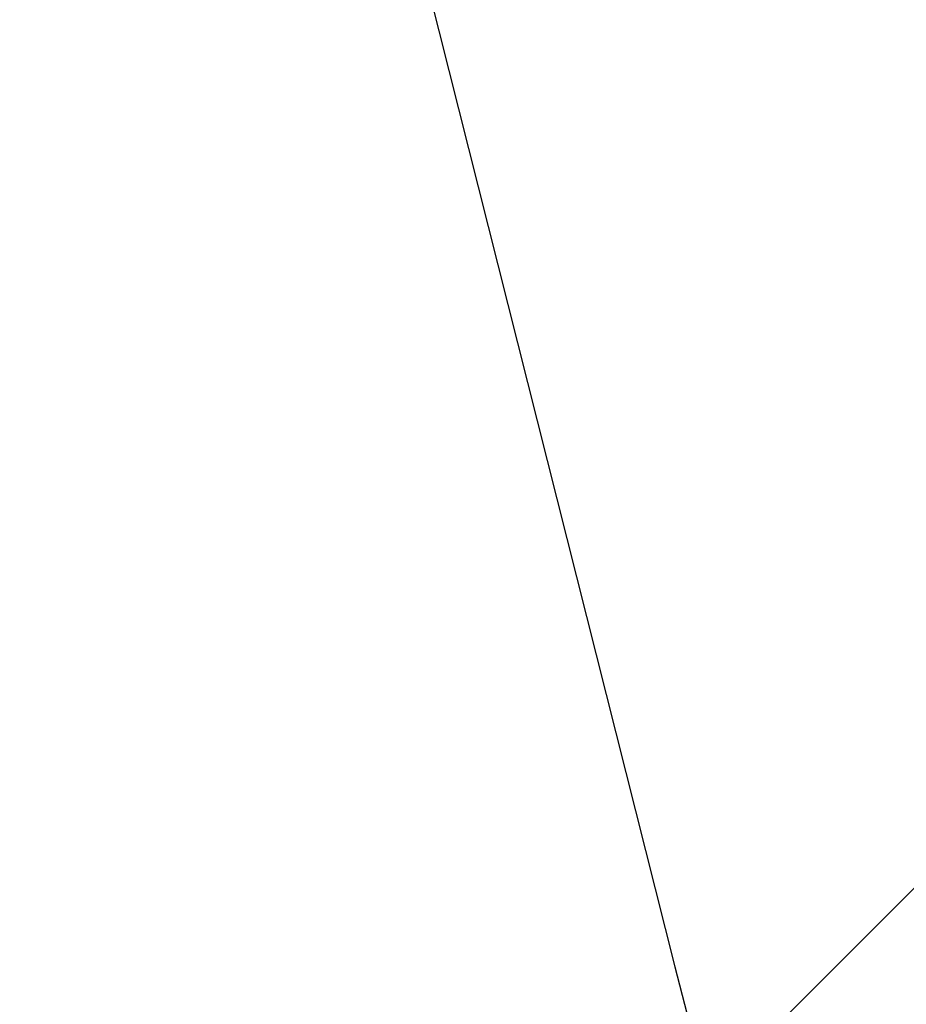
# Model space of a CAD drawing. Units: inches. Extents: x 3590 to 5167, y 65 to 1917.
# Tile 77 of 100: x 5047.497 to 5049.155, y 1787.19 to 1789.032. Entities that reach past the tile are written whole.
import ezdxf

# ---------------------------------------------------------------- set-up
doc = ezdxf.new("R2010")
doc.units = ezdxf.units.IN
for name, color, linetype, lineweight in [('A-ANNO-DIMS', 2, 'Continuous', 18), ('A-FLOR-PATT', 8, 'Continuous', 13), ('L-PLNT', 94, 'Continuous', 18)]:
    doc.layers.add(name, color=color, linetype=linetype, lineweight=lineweight)
doc.layers.add('DIENHOA', color=3, linetype='Continuous')
doc.styles.get("Standard").update_dxf_attribs({"font": 'arial.ttf'})
doc.dimstyles.new('ISO-25', dxfattribs={"dimtxt": 9, "dimasz": 2.5, "dimexe": 1.25, "dimexo": 0.625, "dimtad": 1, "dimdec": 1, "dimlunit": 3, "dimtxsty": 'Standard', "dimcen": 2.5, "dimadec": 0, "dimazin": 0, "dimtfac": 1, "dimtdec": 1, "dimtmove": 0, "dimatfit": 3, "dimfxl": 1, "dimarcsym": 0})

# ---------------------------------------------------------------- blocks, each defined once
blk = doc.blocks.new('Cay03_mb')
at = {"layer": 'DIENHOA'}
blk.add_lwpolyline([(-156.54, 633.124), (-132.463, 551.333), (-110.511, 470.016), (-89.843, 389.218), (-69.618, 308.982), (-48.993, 229.354), (-27.129, 150.379), (-3.182, 72.099), (23.687, -5.439)], dxfattribs=at)
blk = doc.blocks.new('*D322')
at = {"layer": 'A-ANNO-DIMS', "color": 0, "lineweight": -2, "transparency": 16777216}
for p, q in [((5035.7437, 1766.1842), (5035.7437, 1761.199)), ((5064.812, 1766.1842), (5064.812, 1761.199)), ((5038.2437, 1762.449), (5062.312, 1762.449)), ((5064.812, 1762.449), (5166.9911, 1762.449))]:
    blk.add_line(p, q, dxfattribs=at)
at = {"layer": 'A-ANNO-DIMS', "color": 0, "transparency": 16777216}
for points in [[(5038.2437, 1762.8657), (5038.2437, 1762.0323), (5035.7437, 1762.449)], [(5062.312, 1762.8657), (5062.312, 1762.0323), (5064.812, 1762.449)]]:
    blk.add_solid(points, dxfattribs=at)
at = {"layer": 'Defpoints', "color": 0, "transparency": 16777216}
for p in [(5035.7437, 1766.8092), (5064.812, 1766.8092), (5064.812, 1762.449)]:
    blk.add_point(p, dxfattribs=at)
at = {"layer": 'A-ANNO-DIMS', "color": 0, "transparency": 16777216, "insert": (5117.1516, 1767.6692), "char_height": 9, "attachment_point": 5}
blk.add_mtext('PLANT 2\'-5" TYP.', dxfattribs=at)

msp = doc.modelspace()

# ---------------------------------------------------------------- hatches: boundary and pattern name
at = {"layer": 'A-FLOR-PATT', "transparency": 33554687}
h = msp.add_hatch(dxfattribs=at)
h.set_pattern_fill('AR-HBONE', color=256, scale=0.2)
h.set_pattern_definition([(45, (-588.972, 0), (0, 28.73682), [60.96, -20.32]), (135, (-574.604, 14.368), (3e-15, 28.73682), [60.96, -20.32])])
h.paths.add_polyline_path([(5071.274, 1796.999), (4933.274, 1796.999), (4933.274, 1753.999), (4962.774, 1753.999, -0.414214), (4928.774, 1719.999), (4933.274, 1718.999), (4933.274, 1334.999), (5071.274, 1334.999)])
h.paths.add_polyline_path([(4951.78, 1521.0767), (4951.7151, 1521.0404), (4951.5634, 1520.8953)], flags=16)
h.paths.add_polyline_path([(4952.267, 1521.3764), (4952.1977, 1521.3711), (4952.1982, 1521.3556)], flags=0)
h.paths.add_polyline_path([(4967.0508, 1529.7283), (4965.2312, 1528.6944), (4963.4111, 1527.714), (4961.7565, 1526.8508), (4963.5889, 1527.4494), (4964.0356, 1527.478), (4962.9755, 1527.249), (4961.7602, 1526.852), (4959.7922, 1525.8341), (4958.005, 1524.8948), (4956.2403, 1523.9296), (4954.5039, 1522.9185), (4954.1294, 1522.6816), (4953.3605, 1521.9969), (4953.3656, 1521.9975), (4953.605, 1522.0637), (4955.1061, 1522.7608), (4956.9211, 1523.4341), (4958.6778, 1523.9151), (4960.3583, 1524.2004), (4961.9446, 1524.2861), (4964.1714, 1524.1085), (4965.9575, 1523.309), (4963.8627, 1522.9756), (4965.1874, 1522.499), (4963.3661, 1522.4971), (4961.5453, 1522.4868), (4959.7636, 1522.4608), (4958.3041, 1522.4188), (4957.9736, 1522.3883), (4956.3069, 1522.2324), (4954.7182, 1522.0714), (4953.2508, 1521.8992), (4953.5251, 1521.6228), (4954.3309, 1521.3788), (4956.2426, 1521.2299), (4958.0391, 1520.9295), (4959.6842, 1520.4834), (4961.1601, 1519.8957), (4963.107, 1518.8002), (4964.3929, 1517.3252), (4962.9731, 1517.726), (4964.5584, 1516.6606), (4965.4066, 1515.7078), (4963.5073, 1516.3218), (4961.68, 1517.0051), (4959.9348, 1517.7449), (4958.2821, 1518.5283), (4956.7322, 1519.3426), (4955.2953, 1520.1748), (4954.6715, 1520.5724), (4954.5128, 1520.6271), (4955.6585, 1519.3184), (4956.7026, 1517.9823), (4957.644, 1516.6466), (4958.4855, 1515.3344), (4959.55, 1513.524), (4960.4377, 1511.7694), (4958.8411, 1513.6196), (4957.4517, 1515.3249), (4955.8186, 1517.4586), (4956.6654, 1515.4476), (4957.1111, 1513.9229), (4957.4468, 1511.7143), (4957.0764, 1509.7929), (4956.5376, 1511.1103), (4955.9923, 1512.5689), (4955.4445, 1514.1251), (4954.8979, 1515.7352), (4954.3565, 1517.3555), (4953.8241, 1518.9425), (4953.3046, 1520.4525), (4953.0645, 1521.1156), (4952.9714, 1521.1461), (4952.9493, 1521.0865), (4952.7298, 1520.199), (4953.3698, 1518.0236), (4953.7571, 1516.3728), (4954.0512, 1514.7654), (4954.2645, 1513.2212), (4954.4712, 1511.1312), (4954.4971, 1510.4017), (4954.409, 1511.7601), (4954.2645, 1513.2212), (4954.0512, 1514.7654), (4953.7571, 1516.3728), (4953.3698, 1518.0236), (4952.8772, 1519.6981), (4952.7161, 1520.1412), (4952.533, 1519.0587), (4952.3743, 1517.7888), (4952.2192, 1516.3117), (4952.046, 1514.5999), (4951.8325, 1512.626), (4951.557, 1510.3626), (4951.2033, 1512.1682), (4950.8517, 1514.3393), (4950.9853, 1516.3759), (4951.6596, 1518.2862), (4952.5926, 1520.4808), (4952.3566, 1521.1299), (4951.855, 1520.3275), (4950.839, 1518.9083), (4949.7767, 1517.5866), (4948.9155, 1516.6173), (4948.111, 1515.2561), (4947.0891, 1513.5539), (4945.8894, 1511.6149), (4946.3259, 1513.4023), (4946.5624, 1514.2491), (4945.5277, 1513.3267), (4944.5811, 1512.5313), (4946.0177, 1514.5082), (4947.2044, 1516.0476), (4947.8933, 1517.3133), (4949.3069, 1518.7645), (4950.4142, 1519.7672), (4950.4513, 1519.8063), (4952.267, 1521.3764), (4951.6446, 1521.4932), (4950.4037, 1521.1795), (4948.0445, 1520.3587), (4946.1186, 1519.452), (4944.5718, 1518.4748), (4943.3496, 1517.4427), (4941.997, 1515.9197), (4941.6615, 1515.2748), (4942.8133, 1516.9897), (4944.5718, 1518.4748), (4946.1186, 1519.452), (4948.0445, 1520.3587), (4950.4037, 1521.1795), (4951.6446, 1521.4932), (4949.6468, 1521.8678), (4948.5998, 1521.7563), (4947.1263, 1521.5699), (4945.4202, 1521.3476), (4943.4497, 1521.1046), (4941.1832, 1520.856), (4942.8603, 1521.6126), (4943.8731, 1522.0301), (4942.9522, 1521.9093), (4941.4097, 1521.4851), (4939.5429, 1520.6702), (4938.9677, 1520.2255), (4940.7328, 1521.299), (4942.9522, 1521.9093), (4943.7018, 1522.0077), (4945.8942, 1522.7), (4947.5649, 1522.714), (4948.9209, 1522.5657), (4951.1314, 1522.1827), (4950.9706, 1522.2969), (4948.1292, 1523.0056), (4946.035, 1523.7067), (4944.2323, 1524.5214), (4942.7069, 1525.4611), (4941.4442, 1526.5371), (4940.4297, 1527.7606), (4939.6489, 1529.1431), (4941.4209, 1528.1223), (4943.1474, 1527.1325), (4944.8409, 1526.1746), (4946.5139, 1525.2496), (4948.1789, 1524.3586), (4948.3646, 1524.2634), (4946.4753, 1526.0446), (4945.1808, 1527.5404), (4944.1904, 1529.0334), (4943.4956, 1530.5398), (4943.2781, 1531.3597), (4942.4985, 1531.919), (4943.1135, 1531.7625), (4942.9593, 1533.6586), (4944.1395, 1531.9886), (4944.6117, 1531.3234), (4946.2016, 1530.4634), (4947.4857, 1529.5093), (4948.7903, 1528.2265), (4950.3675, 1526.2375), (4949.4855, 1528.1555), (4948.8513, 1530.1225), (4948.4905, 1532.0413), (4948.3811, 1533.9182), (4948.5006, 1535.7599), (4948.827, 1537.5728), (4949.418, 1535.5653), (4949.9568, 1533.5693), (4950.4641, 1531.5861), (4950.9606, 1529.6167), (4951.3911, 1527.9545), (4951.7235, 1530.6869), (4952.2011, 1532.5799), (4952.8891, 1534.3296), (4953.7703, 1535.9512), (4954.8273, 1537.46), (4954.5214, 1535.3897), (4954.2731, 1533.9368), (4955.58, 1535.6627), (4956.7476, 1536.7386), (4956.1585, 1534.7803), (4955.5892, 1532.8733), (4955.0434, 1531.0058), (4954.5249, 1529.1658), (4954.0377, 1527.3413), (4953.6383, 1525.733), (4953.6114, 1525.5856), (4953.3981, 1524.1657), (4953.3822, 1524.0089), (4954.0696, 1525.4756), (4954.9121, 1527.0217), (4956.1363, 1528.8935), (4957.8467, 1530.577), (4959.376, 1531.5401), (4958.256, 1530.104), (4957.1428, 1528.6629), (4956.0663, 1527.2431), (4955.0558, 1525.8705), (4954.141, 1524.5715), (4953.3516, 1523.372), (4953.3108, 1523.303), (4953.2725, 1522.9248), (4953.261, 1522.3821), (4954.1031, 1523.3727), (4954.63, 1524.2838), (4955.9615, 1526.3577), (4957.23, 1528.1297), (4958.4206, 1529.6086), (4960.0367, 1531.3679), (4961.3736, 1532.3752), (4962.1015, 1532.77), (4961.0699, 1531.0611), (4959.9873, 1529.4381), (4958.8685, 1527.908), (4958.1505, 1527.0074), (4959.8029, 1528.0031), (4961.5885, 1528.7926), (4963.3909, 1529.3278), (4965.2112, 1529.6321)], flags=16)
h.paths.add_polyline_path([(4962.9439, 1523.1819), (4961.1071, 1523.4219), (4960.3921, 1523.3616), (4962.3496, 1523.3306)], flags=0)
h.paths.add_polyline_path([(5049.5413, 1584.5509), (5049.4764, 1584.5146), (5049.3247, 1584.3695)], flags=16)
h.paths.add_polyline_path([(5050.0283, 1584.8506), (5049.959, 1584.8453), (5049.9595, 1584.8298)], flags=0)
h.paths.add_polyline_path([(5042.3331, 1581.949), (5043.8799, 1582.9262), (5045.8057, 1583.8329), (5048.165, 1584.6537), (5049.4058, 1584.9674), (5047.408, 1585.342), (5046.3611, 1585.2305), (5044.8876, 1585.0441), (5043.1814, 1584.8218), (5041.211, 1584.5788), (5038.9445, 1584.3301), (5040.6215, 1585.0868), (5041.6343, 1585.5043), (5040.7134, 1585.3835), (5039.1709, 1584.9593), (5037.3041, 1584.1444), (5036.729, 1583.6997), (5038.4941, 1584.7732), (5040.7134, 1585.3835), (5041.4631, 1585.4819), (5043.6555, 1586.1742), (5045.3261, 1586.1882), (5046.6821, 1586.0399), (5048.8927, 1585.6569), (5048.7319, 1585.7711), (5045.8905, 1586.4798), (5043.7962, 1587.1809), (5041.9936, 1587.9956), (5040.4682, 1588.9353), (5039.2055, 1590.0113), (5038.1909, 1591.2348), (5037.4102, 1592.6172), (5039.1822, 1591.5965), (5040.9087, 1590.6067), (5042.6022, 1589.6488), (5044.2752, 1588.7238), (5045.9402, 1587.8327), (5046.1258, 1587.7375), (5044.2366, 1589.5188), (5042.9421, 1591.0146), (5041.9517, 1592.5076), (5041.2569, 1594.014), (5041.0393, 1594.8339), (5040.2598, 1595.3932), (5040.8748, 1595.2367), (5040.7205, 1597.1328), (5041.9008, 1595.4628), (5042.373, 1594.7976), (5043.9629, 1593.9376), (5045.2469, 1592.9834), (5046.5515, 1591.7007), (5048.1288, 1589.7116), (5047.2467, 1591.6297), (5046.6125, 1593.5967), (5046.2518, 1595.5155), (5046.1423, 1597.3924), (5046.2619, 1599.2341), (5046.5883, 1601.047), (5047.1793, 1599.0394), (5047.7181, 1597.0435), (5048.2254, 1595.0603), (5048.7218, 1593.0909), (5049.1524, 1591.4287), (5049.4848, 1594.1611), (5049.9623, 1596.0541), (5050.6504, 1597.8038), (5051.5316, 1599.4254), (5052.5885, 1600.9341), (5052.2827, 1598.8638), (5052.0344, 1597.411), (5053.3413, 1599.1369), (5054.5088, 1600.2128), (5053.9198, 1598.2545), (5053.3504, 1596.3475), (5052.8046, 1594.48), (5052.2862, 1592.6399), (5051.799, 1590.8155), (5051.3996, 1589.2072), (5051.3727, 1589.0598), (5051.1593, 1587.6398), (5051.1435, 1587.4831), (5051.8308, 1588.9498), (5052.6734, 1590.4959), (5053.8975, 1592.3677), (5055.6079, 1594.0512), (5057.1373, 1595.0143), (5056.0172, 1593.5782), (5054.9041, 1592.1371), (5053.8275, 1590.7172), (5052.8171, 1589.3447), (5051.9023, 1588.0457), (5051.1129, 1586.8462), (5051.0721, 1586.7772), (5051.0338, 1586.399), (5051.0223, 1585.8563), (5051.8644, 1586.8469), (5052.3913, 1587.7579), (5053.7228, 1589.8318), (5054.9913, 1591.6039), (5056.1818, 1593.0828), (5057.798, 1594.8421), (5059.1349, 1595.8494), (5059.8628, 1596.2442), (5058.8312, 1594.5353), (5057.7486, 1592.9123), (5056.6298, 1591.3822), (5055.9117, 1590.4816), (5057.5642, 1591.4773), (5059.3498, 1592.2667), (5061.1521, 1592.802), (5062.9724, 1593.1062), (5064.812, 1593.2025), (5062.9925, 1592.1686), (5061.1724, 1591.1882), (5059.5178, 1590.325), (5061.3501, 1590.9236), (5061.7968, 1590.9522), (5060.7368, 1590.7232), (5059.5215, 1590.3262), (5057.5535, 1589.3082), (5055.7662, 1588.369), (5054.0016, 1587.4038), (5052.2652, 1586.3927), (5051.8907, 1586.1558), (5051.1218, 1585.4711), (5051.1268, 1585.4717), (5051.3663, 1585.5379), (5052.8673, 1586.235), (5054.6823, 1586.9082), (5056.4391, 1587.3893), (5058.1196, 1587.6745), (5059.7058, 1587.7602), (5061.9327, 1587.5827), (5063.7188, 1586.7832), (5061.624, 1586.4498), (5062.9487, 1585.9732), (5061.1274, 1585.9713), (5059.3065, 1585.961), (5057.5249, 1585.935), (5056.0654, 1585.893), (5055.7348, 1585.8625), (5054.0682, 1585.7066), (5052.4795, 1585.5456), (5051.012, 1585.3733), (5051.2864, 1585.097), (5052.0921, 1584.853), (5054.0039, 1584.7041), (5055.8004, 1584.4037), (5057.4455, 1583.9576), (5058.9213, 1583.3699), (5060.8683, 1582.2744), (5062.1541, 1580.7994), (5060.7343, 1581.2001), (5062.3197, 1580.1348), (5063.1679, 1579.182), (5061.2686, 1579.796), (5059.4412, 1580.4793), (5057.696, 1581.2191), (5056.0434, 1582.0025), (5054.4934, 1582.8168), (5053.0565, 1583.649), (5052.4328, 1584.0466), (5052.2741, 1584.1013), (5053.4197, 1582.7925), (5054.4639, 1581.4565), (5055.4053, 1580.1208), (5056.2467, 1578.8086), (5057.3112, 1576.9982), (5058.1989, 1575.2435), (5056.6023, 1577.0938), (5055.213, 1578.7991), (5053.5799, 1580.9327), (5054.4266, 1578.9218), (5054.8724, 1577.3971), (5055.2081, 1575.1885), (5054.8377, 1573.2671), (5054.2988, 1574.5845), (5053.7536, 1576.0431), (5053.2057, 1577.5993), (5052.6592, 1579.2094), (5052.1178, 1580.8297), (5051.5854, 1582.4167), (5051.0658, 1583.9267), (5050.8258, 1584.5898), (5050.7327, 1584.6203), (5050.7106, 1584.5606), (5050.4911, 1583.6732), (5051.1311, 1581.4978), (5051.5183, 1579.847), (5051.8125, 1578.2396), (5052.0257, 1576.6954), (5052.2325, 1574.6054), (5052.2584, 1573.8759), (5052.1703, 1575.2342), (5052.0257, 1576.6954), (5051.8125, 1578.2396), (5051.5183, 1579.847), (5051.1311, 1581.4978), (5050.6384, 1583.1723), (5050.4774, 1583.6154), (5050.2943, 1582.5329), (5050.1355, 1581.263), (5049.9805, 1579.7859), (5049.8072, 1578.074), (5049.5938, 1576.1002), (5049.3182, 1573.8368), (5048.9646, 1575.6424), (5048.6129, 1577.8135), (5048.7466, 1579.8501), (5049.4209, 1581.7604), (5050.3539, 1583.955), (5050.1179, 1584.6041), (5049.6163, 1583.8017), (5048.6003, 1582.3825), (5047.538, 1581.0608), (5046.6768, 1580.0915), (5045.8722, 1578.7303), (5044.8504, 1577.0281), (5043.6506, 1575.0891), (5044.0871, 1576.8765), (5044.3237, 1577.7233), (5043.289, 1576.8009), (5042.3423, 1576.0054), (5043.779, 1577.9824), (5044.9657, 1579.5218), (5045.6546, 1580.7875), (5047.0681, 1582.2386), (5048.1754, 1583.2413), (5048.2126, 1583.2805), (5050.0283, 1584.8506), (5049.4058, 1584.9674), (5048.165, 1584.6537), (5045.8057, 1583.8329), (5043.8799, 1582.9262), (5042.3331, 1581.949), (5041.1109, 1580.9168), (5039.7582, 1579.3939), (5039.4227, 1578.7489), (5040.5746, 1580.4639)], flags=16)
h.paths.add_polyline_path([(4954.7987, 1533.1203), (4954.2625, 1532.0793), (4953.8311, 1530.9346), (4953.5047, 1529.636), (4953.2834, 1528.1333), (4953.1672, 1526.3764), (4953.1563, 1524.315), (4953.2767, 1521.2363), (4952.8017, 1521.8418), (4951.557, 1521.9979), (4950.9758, 1521.9613), (4952.6606, 1521.941), (4952.8017, 1521.8418), (4953.1525, 1523.5926), (4953.1672, 1526.3764), (4953.2834, 1528.1333), (4953.6093, 1530.346), (4954.4556, 1532.5917)], flags=0)
h.paths.add_polyline_path([(5050.5629, 1585.316), (5049.3182, 1585.4721), (5048.737, 1585.4355), (5050.4219, 1585.4152), (5050.5629, 1585.316), (5050.9138, 1587.0668), (5050.9285, 1589.8506), (5051.0446, 1591.6075), (5051.3706, 1593.8202), (5052.2168, 1596.0659), (5052.56, 1596.5945), (5052.0238, 1595.5535), (5051.5924, 1594.4088), (5051.266, 1593.1102), (5051.0446, 1591.6075), (5050.9285, 1589.8506), (5050.9176, 1587.7892), (5051.038, 1584.7105)], flags=0)
h.paths.add_polyline_path([(5058.1533, 1586.8358), (5060.1109, 1586.8048), (5060.7051, 1586.6561), (5058.8684, 1586.8961)], flags=0)
h.paths.add_polyline_path([(5049.5413, 1430.9361), (5049.4764, 1430.8998), (5049.3247, 1430.7547)], flags=16)
h.paths.add_polyline_path([(5050.0283, 1431.2359), (5049.959, 1431.2305), (5049.9595, 1431.215)], flags=0)
h.paths.add_polyline_path([(5046.5883, 1447.4322), (5047.1793, 1445.4247), (5047.7181, 1443.4287), (5048.2254, 1441.4455), (5048.7218, 1439.4761), (5049.1524, 1437.8139), (5049.4848, 1440.5463), (5049.9623, 1442.4393), (5050.6504, 1444.189), (5051.5316, 1445.8106), (5052.5885, 1447.3194), (5052.2827, 1445.2491), (5052.0344, 1443.7962), (5053.3413, 1445.5221), (5054.5088, 1446.598), (5053.9198, 1444.6397), (5053.3504, 1442.7327), (5052.8046, 1440.8652), (5052.2862, 1439.0252), (5051.799, 1437.2007), (5051.3996, 1435.5924), (5051.3727, 1435.445), (5051.1593, 1434.0251), (5051.1435, 1433.8683), (5051.8308, 1435.335), (5052.6734, 1436.8811), (5053.8975, 1438.7529), (5055.6079, 1440.4364), (5057.1373, 1441.3995), (5056.0172, 1439.9634), (5054.9041, 1438.5223), (5053.8275, 1437.1025), (5052.8171, 1435.7299), (5051.9023, 1434.4309), (5051.1129, 1433.2314), (5051.0721, 1433.1624), (5051.0338, 1432.7842), (5051.0223, 1432.2415), (5051.8644, 1433.2321), (5052.3913, 1434.1432), (5053.7228, 1436.2171), (5054.9913, 1437.9891), (5056.1818, 1439.468), (5057.798, 1441.2273), (5059.1349, 1442.2346), (5059.8628, 1442.6294), (5058.8312, 1440.9205), (5057.7486, 1439.2975), (5056.6298, 1437.7674), (5055.9117, 1436.8668), (5057.5642, 1437.8625), (5059.3498, 1438.652), (5061.1521, 1439.1872), (5062.9724, 1439.4915), (5064.812, 1439.5877), (5062.9925, 1438.5538), (5061.1724, 1437.5734), (5059.5178, 1436.7102), (5061.3501, 1437.3088), (5061.7968, 1437.3374), (5060.7368, 1437.1084), (5059.5215, 1436.7114), (5057.5535, 1435.6935), (5055.7662, 1434.7542), (5054.0016, 1433.789), (5052.2652, 1432.7779), (5051.8907, 1432.541), (5051.1218, 1431.8563), (5051.1268, 1431.8569), (5051.3663, 1431.9231), (5052.8673, 1432.6202), (5054.6823, 1433.2935), (5056.4391, 1433.7745), (5058.1196, 1434.0598), (5059.7058, 1434.1455), (5061.9327, 1433.9679), (5063.7188, 1433.1684), (5061.624, 1432.8351), (5062.9487, 1432.3584), (5061.1274, 1432.3566), (5059.3065, 1432.3462), (5057.5249, 1432.3202), (5056.0654, 1432.2782), (5055.7348, 1432.2477), (5054.0682, 1432.0918), (5052.4795, 1431.9308), (5051.012, 1431.7586), (5051.2864, 1431.4822), (5052.0921, 1431.2382), (5054.0039, 1431.0893), (5055.8004, 1430.7889), (5057.4455, 1430.3428), (5058.9213, 1429.7551), (5060.8683, 1428.6596), (5062.1541, 1427.1846), (5060.7343, 1427.5854), (5062.3197, 1426.52), (5063.1679, 1425.5672), (5061.2686, 1426.1812), (5059.4412, 1426.8645), (5057.696, 1427.6043), (5056.0434, 1428.3877), (5054.4934, 1429.202), (5053.0565, 1430.0342), (5052.4328, 1430.4318), (5052.2741, 1430.4865), (5053.4197, 1429.1778), (5054.4639, 1427.8417), (5055.4053, 1426.506), (5056.2467, 1425.1938), (5057.3112, 1423.3834), (5058.1989, 1421.6288), (5056.6023, 1423.479), (5055.213, 1425.1843), (5053.5799, 1427.318), (5054.4266, 1425.307), (5054.8724, 1423.7823), (5055.2081, 1421.5737), (5054.8377, 1419.6523), (5054.2988, 1420.9697), (5053.7536, 1422.4283), (5053.2057, 1423.9845), (5052.6592, 1425.5946), (5052.1178, 1427.2149), (5051.5854, 1428.8019), (5051.0658, 1430.3119), (5050.8258, 1430.975), (5050.7327, 1431.0055), (5050.7106, 1430.9459), (5050.4911, 1430.0585), (5051.1311, 1427.883), (5051.5183, 1426.2322), (5051.8125, 1424.6248), (5052.0257, 1423.0806), (5052.2325, 1420.9906), (5052.2584, 1420.2611), (5052.1703, 1421.6195), (5052.0257, 1423.0806), (5051.8125, 1424.6248), (5051.5183, 1426.2322), (5051.1311, 1427.883), (5050.6384, 1429.5575), (5050.4774, 1430.0006), (5050.2943, 1428.9181), (5050.1355, 1427.6482), (5049.9805, 1426.1711), (5049.8072, 1424.4593), (5049.5938, 1422.4854), (5049.3182, 1420.222), (5048.9646, 1422.0276), (5048.6129, 1424.1987), (5048.7466, 1426.2353), (5049.4209, 1428.1457), (5050.3539, 1430.3403), (5050.1179, 1430.9893), (5049.6163, 1430.1869), (5048.6003, 1428.7677), (5047.538, 1427.446), (5046.6768, 1426.4767), (5045.8722, 1425.1155), (5044.8504, 1423.4133), (5043.6506, 1421.4744), (5044.0871, 1423.2617), (5044.3237, 1424.1085), (5043.289, 1423.1861), (5042.3423, 1422.3907), (5043.779, 1424.3677), (5044.9657, 1425.907), (5045.6546, 1427.1727), (5047.0681, 1428.6239), (5048.1754, 1429.6266), (5048.2126, 1429.6657), (5050.0283, 1431.2359), (5049.4058, 1431.3526), (5048.165, 1431.0389), (5045.8057, 1430.2181), (5043.8799, 1429.3114), (5042.3331, 1428.3342), (5041.1109, 1427.3021), (5039.7582, 1425.7791), (5039.4227, 1425.1342), (5040.5746, 1426.8491), (5042.3331, 1428.3342), (5043.8799, 1429.3114), (5045.8057, 1430.2181), (5048.165, 1431.0389), (5049.4058, 1431.3526), (5047.408, 1431.7272), (5046.3611, 1431.6157), (5044.8876, 1431.4293), (5043.1814, 1431.207), (5041.211, 1430.964), (5038.9445, 1430.7154), (5040.6215, 1431.4721), (5041.6343, 1431.8895), (5040.7134, 1431.7687), (5039.1709, 1431.3445), (5037.3041, 1430.5296), (5036.729, 1430.0849), (5038.4941, 1431.1584), (5040.7134, 1431.7687), (5041.4631, 1431.8671), (5043.6555, 1432.5594), (5045.3261, 1432.5734), (5046.6821, 1432.4251), (5048.8927, 1432.0421), (5048.7319, 1432.1563), (5045.8905, 1432.865), (5043.7962, 1433.5661), (5041.9936, 1434.3808), (5040.4682, 1435.3205), (5039.2055, 1436.3965), (5038.1909, 1437.62), (5037.4102, 1439.0025), (5039.1822, 1437.9817), (5040.9087, 1436.9919), (5042.6022, 1436.034), (5044.2752, 1435.109), (5045.9402, 1434.218), (5046.1258, 1434.1228), (5044.2366, 1435.904), (5042.9421, 1437.3998), (5041.9517, 1438.8928), (5041.2569, 1440.3993), (5041.0393, 1441.2191), (5040.2598, 1441.7784), (5040.8748, 1441.6219), (5040.7205, 1443.518), (5041.9008, 1441.848), (5042.373, 1441.1828), (5043.9629, 1440.3228), (5045.2469, 1439.3687), (5046.5515, 1438.0859), (5048.1288, 1436.0969), (5047.2467, 1438.0149), (5046.6125, 1439.9819), (5046.2518, 1441.9007), (5046.1423, 1443.7776), (5046.2619, 1445.6193)], flags=16)
h.paths.add_polyline_path([(5052.3818, 1444.255), (5051.6226, 1442.7799), (5052.0238, 1441.9388), (5052.56, 1442.9797)], flags=0)
h.paths.add_polyline_path([(5050.5629, 1431.7012), (5049.3182, 1431.8573), (5048.737, 1431.8207), (5050.4219, 1431.8004)], flags=0)
h.paths.add_polyline_path([(5058.1533, 1433.221), (5060.1109, 1433.19), (5060.7051, 1433.0413), (5058.8684, 1433.2813)], flags=0)
h.paths.add_polyline_path([(5049.5413, 1352.2853), (5049.4764, 1352.249), (5049.3247, 1352.104)], flags=16)
h.paths.add_polyline_path([(5050.0283, 1352.5851), (5049.959, 1352.5797), (5049.9595, 1352.5642)], flags=0)
h.paths.add_polyline_path([(5046.5883, 1368.7815), (5047.1793, 1366.7739), (5047.7181, 1364.778), (5048.2254, 1362.7947), (5048.7218, 1360.8253), (5049.1524, 1359.1631), (5049.4848, 1361.8955), (5049.9623, 1363.7886), (5050.6504, 1365.5383), (5051.5316, 1367.1599), (5052.5885, 1368.6686), (5052.2827, 1366.5983), (5052.0344, 1365.1455), (5053.3413, 1366.8713), (5054.5088, 1367.9472), (5053.9198, 1365.9889), (5053.3504, 1364.082), (5052.8046, 1362.2144), (5052.2862, 1360.3744), (5051.799, 1358.5499), (5051.3996, 1356.9416), (5051.3727, 1356.7943), (5051.1593, 1355.3743), (5051.1435, 1355.2175), (5051.8308, 1356.6843), (5052.6734, 1358.2304), (5053.8975, 1360.1022), (5055.6079, 1361.7857), (5057.1373, 1362.7488), (5056.0172, 1361.3126), (5054.9041, 1359.8716), (5053.8275, 1358.4517), (5052.8171, 1357.0792), (5051.9023, 1355.7801), (5051.1129, 1354.5807), (5051.0721, 1354.5116), (5051.0338, 1354.1334), (5051.0223, 1353.5908), (5051.8644, 1354.5814), (5052.3913, 1355.4924), (5053.7228, 1357.5663), (5054.9913, 1359.3383), (5056.1818, 1360.8173), (5057.798, 1362.5766), (5059.1349, 1363.5838), (5059.8628, 1363.9786), (5058.8312, 1362.2698), (5057.7486, 1360.6468), (5056.6298, 1359.1167), (5055.9117, 1358.2161), (5057.5642, 1359.2118), (5059.3498, 1360.0012), (5061.1521, 1360.5365), (5062.9724, 1360.8407), (5064.812, 1360.937), (5062.9925, 1359.9031), (5061.1724, 1358.9227), (5059.5178, 1358.0595), (5061.3501, 1358.658), (5061.7968, 1358.6867), (5060.7368, 1358.4577), (5059.5215, 1358.0607), (5057.5535, 1357.0427), (5055.7662, 1356.1035), (5054.0016, 1355.1382), (5052.2652, 1354.1272), (5051.8907, 1353.8903), (5051.1218, 1353.2055), (5051.1268, 1353.2062), (5051.3663, 1353.2723), (5052.8673, 1353.9695), (5054.6823, 1354.6427), (5056.4391, 1355.1238), (5058.1196, 1355.409), (5059.7058, 1355.4947), (5061.9327, 1355.3171), (5063.7188, 1354.5177), (5061.624, 1354.1843), (5062.9487, 1353.7076), (5061.1274, 1353.7058), (5059.3065, 1353.6955), (5057.5249, 1353.6694), (5056.0654, 1353.6274), (5055.7348, 1353.5969), (5054.0682, 1353.441), (5052.4795, 1353.2801), (5051.012, 1353.1078), (5051.2864, 1352.8314), (5052.0921, 1352.5875), (5054.0039, 1352.4385), (5055.8004, 1352.1382), (5057.4455, 1351.692), (5058.9213, 1351.1043), (5060.8683, 1350.0089), (5062.1541, 1348.5338), (5060.7343, 1348.9346), (5062.3197, 1347.8692), (5063.1679, 1346.9164), (5061.2686, 1347.5304), (5059.4412, 1348.2137), (5057.696, 1348.9535), (5056.0434, 1349.737), (5054.4934, 1350.5512), (5053.0565, 1351.3834), (5052.4328, 1351.781), (5052.2741, 1351.8357), (5053.4197, 1350.527), (5054.4639, 1349.191), (5055.4053, 1347.8553), (5056.2467, 1346.543), (5057.3112, 1344.7326), (5058.1989, 1342.978), (5056.6023, 1344.8282), (5055.213, 1346.5335), (5053.5799, 1348.6672), (5054.4266, 1346.6563), (5054.8724, 1345.1316), (5055.2081, 1342.923), (5054.8377, 1341.0015), (5054.2988, 1342.3189), (5053.7536, 1343.7776), (5053.2057, 1345.3337), (5052.6592, 1346.9438), (5052.1178, 1348.5642), (5051.5854, 1350.1512), (5051.0658, 1351.6611), (5050.8258, 1352.3243), (5050.7327, 1352.3547), (5050.7106, 1352.2951), (5050.4911, 1351.4077), (5051.1311, 1349.2323), (5051.5183, 1347.5814), (5051.8125, 1345.974), (5052.0257, 1344.4298), (5052.2325, 1342.3399), (5052.2584, 1341.6104), (5052.1703, 1342.9687), (5052.0257, 1344.4298), (5051.8125, 1345.974), (5051.5183, 1347.5814), (5051.1311, 1349.2323), (5050.6384, 1350.9068), (5050.4774, 1351.3498), (5050.2943, 1350.2674), (5050.1355, 1348.9975), (5049.9805, 1347.5203), (5049.8072, 1345.8085), (5049.5938, 1343.8346), (5049.3182, 1341.5712), (5048.9646, 1343.3768), (5048.6129, 1345.548), (5048.7466, 1347.5846), (5049.4209, 1349.4949), (5050.3539, 1351.6895), (5050.1179, 1352.3385), (5049.6163, 1351.5362), (5048.6003, 1350.1169), (5047.538, 1348.7952), (5046.6768, 1347.826), (5045.8722, 1346.4647), (5044.8504, 1344.7625), (5043.6506, 1342.8236), (5044.0871, 1344.611), (5044.3237, 1345.4578), (5043.289, 1344.5353), (5042.3423, 1343.7399), (5043.779, 1345.7169), (5044.9657, 1347.2563), (5045.6546, 1348.522), (5047.0681, 1349.9731), (5048.1754, 1350.9758), (5048.2126, 1351.0149), (5050.0283, 1352.5851), (5049.4058, 1352.7018), (5048.165, 1352.3882), (5045.8057, 1351.5673), (5043.8799, 1350.6606), (5042.3331, 1349.6835), (5041.1109, 1348.6513), (5039.7582, 1347.1283), (5039.4227, 1346.4834), (5040.5746, 1348.1984), (5042.3331, 1349.6835), (5043.8799, 1350.6606), (5045.8057, 1351.5673), (5048.165, 1352.3882), (5049.4058, 1352.7018), (5047.408, 1353.0765), (5046.3611, 1352.965), (5044.8876, 1352.7785), (5043.1814, 1352.5563), (5041.211, 1352.3133), (5038.9445, 1352.0646), (5040.6215, 1352.8213), (5041.6343, 1353.2388), (5040.7134, 1353.1179), (5039.1709, 1352.6938), (5037.3041, 1351.8788), (5036.729, 1351.4341), (5038.4941, 1352.5076), (5040.7134, 1353.1179), (5041.4631, 1353.2163), (5043.6555, 1353.9086), (5045.3261, 1353.9226), (5046.6821, 1353.7744), (5048.8927, 1353.3914), (5048.7319, 1353.5055), (5045.8905, 1354.2143), (5043.7962, 1354.9153), (5041.9936, 1355.7301), (5040.4682, 1356.6698), (5039.2055, 1357.7457), (5038.1909, 1358.9693), (5037.4102, 1360.3517), (5039.1822, 1359.331), (5040.9087, 1358.3411), (5042.6022, 1357.3832), (5044.2752, 1356.4582), (5045.9402, 1355.5672), (5046.1258, 1355.472), (5044.2366, 1357.2532), (5042.9421, 1358.7491), (5041.9517, 1360.242), (5041.2569, 1361.7485), (5041.0393, 1362.5683), (5040.2598, 1363.1277), (5040.8748, 1362.9711), (5040.7205, 1364.8672), (5041.9008, 1363.1972), (5042.373, 1362.532), (5043.9629, 1361.6721), (5045.2469, 1360.7179), (5046.5515, 1359.4351), (5048.1288, 1357.4461), (5047.2467, 1359.3641), (5046.6125, 1361.3312), (5046.2518, 1363.2499), (5046.1423, 1365.1269), (5046.2619, 1366.9685)], flags=16)
h.paths.add_polyline_path([(5052.3818, 1365.6042), (5051.6226, 1364.1291), (5052.0238, 1363.288), (5052.56, 1364.3289)], flags=0)
h.paths.add_polyline_path([(4951.78, 1698.0408), (4951.7151, 1698.0045), (4951.5634, 1697.8594)], flags=16)
h.paths.add_polyline_path([(4952.267, 1698.3406), (4952.1977, 1698.3352), (4952.1982, 1698.3197)], flags=0)
h.paths.add_polyline_path([(4957.0764, 1686.757), (4956.5376, 1688.0744), (4955.9923, 1689.533), (4955.4445, 1691.0892), (4954.8979, 1692.6993), (4954.3565, 1694.3196), (4953.8241, 1695.9066), (4953.3046, 1697.4166), (4953.0645, 1698.0797), (4952.9714, 1698.1102), (4952.9493, 1698.0506), (4952.7298, 1697.1632), (4953.3698, 1694.9877), (4953.7571, 1693.3369), (4954.0512, 1691.7295), (4954.2645, 1690.1853), (4954.4712, 1688.0953), (4954.4971, 1687.3658), (4954.409, 1688.7242), (4954.2645, 1690.1853), (4954.0512, 1691.7295), (4953.7571, 1693.3369), (4953.3698, 1694.9877), (4952.8772, 1696.6622), (4952.7161, 1697.1053), (4952.533, 1696.0228), (4952.3743, 1694.7529), (4952.2192, 1693.2758), (4952.046, 1691.564), (4951.8325, 1689.5901), (4951.557, 1687.3267), (4951.2033, 1689.1323), (4950.8517, 1691.3034), (4950.9853, 1693.34), (4951.6596, 1695.2504), (4952.5926, 1697.445), (4952.3566, 1698.094), (4951.855, 1697.2916), (4950.839, 1695.8724), (4949.7767, 1694.5507), (4948.9155, 1693.5814), (4948.111, 1692.2202), (4947.0891, 1690.518), (4945.8894, 1688.5791), (4946.3259, 1690.3664), (4946.5624, 1691.2132), (4945.5277, 1690.2908), (4944.5811, 1689.4954), (4946.0177, 1691.4724), (4947.2044, 1693.0117), (4947.8933, 1694.2774), (4949.3069, 1695.7286), (4950.4142, 1696.7313), (4950.4513, 1696.7704), (4952.267, 1698.3406), (4951.6446, 1698.4573), (4950.4037, 1698.1436), (4948.0445, 1697.3228), (4946.1186, 1696.4161), (4944.5718, 1695.4389), (4943.3496, 1694.4068), (4941.997, 1692.8838), (4941.6615, 1692.2389), (4942.8133, 1693.9538), (4944.5718, 1695.4389), (4946.1186, 1696.4161), (4948.0445, 1697.3228), (4950.4037, 1698.1436), (4951.6446, 1698.4573), (4949.6468, 1698.8319), (4948.5998, 1698.7204), (4947.1263, 1698.534), (4945.4202, 1698.3117), (4943.4497, 1698.0687), (4941.1832, 1697.8201), (4942.8603, 1698.5768), (4943.8731, 1698.9942), (4942.9522, 1698.8734), (4941.4097, 1698.4492), (4939.5429, 1697.6343), (4938.9677, 1697.1896), (4940.7328, 1698.2631), (4942.9522, 1698.8734), (4943.7018, 1698.9718), (4945.8942, 1699.6641), (4947.5649, 1699.6781), (4948.9209, 1699.5298), (4951.1314, 1699.1468), (4950.9706, 1699.261), (4948.1292, 1699.9697), (4946.035, 1700.6708), (4944.2323, 1701.4855), (4942.7069, 1702.4252), (4941.4442, 1703.5012), (4940.4297, 1704.7247), (4939.6489, 1706.1072), (4941.4209, 1705.0864), (4943.1474, 1704.0966), (4944.8409, 1703.1387), (4946.5139, 1702.2137), (4948.1789, 1701.3227), (4948.3646, 1701.2275), (4946.4753, 1703.0087), (4945.1808, 1704.5045), (4944.1904, 1705.9975), (4943.4956, 1707.504), (4943.2781, 1708.3238), (4942.4985, 1708.8831), (4943.1135, 1708.7266), (4942.9593, 1710.6227), (4944.1395, 1708.9527), (4944.6117, 1708.2875), (4946.2016, 1707.4275), (4947.4857, 1706.4734), (4948.7903, 1705.1906), (4950.3675, 1703.2016), (4949.4855, 1705.1196), (4948.8513, 1707.0866), (4948.4905, 1709.0054), (4948.3811, 1710.8823), (4948.5006, 1712.724), (4948.827, 1714.5369), (4949.418, 1712.5294), (4949.9568, 1710.5334), (4950.4641, 1708.5502), (4950.9606, 1706.5808), (4951.3911, 1704.9186), (4951.7235, 1707.651), (4952.2011, 1709.544), (4952.8891, 1711.2937), (4953.7703, 1712.9153), (4954.8273, 1714.4241), (4954.5214, 1712.3538), (4954.2731, 1710.9009), (4955.58, 1712.6268), (4956.7476, 1713.7027), (4956.1585, 1711.7444), (4955.5892, 1709.8374), (4955.0434, 1707.9699), (4954.5249, 1706.1299), (4954.0377, 1704.3054), (4953.6383, 1702.6971), (4953.6114, 1702.5497), (4953.3981, 1701.1298), (4953.3822, 1700.973), (4954.0696, 1702.4397), (4954.9121, 1703.9858), (4956.1363, 1705.8576), (4957.8467, 1707.5411), (4959.376, 1708.5042), (4958.256, 1707.0681), (4957.1428, 1705.627), (4956.0663, 1704.2072), (4955.0558, 1702.8346), (4954.141, 1701.5356), (4953.3516, 1700.3361), (4953.3108, 1700.2671), (4953.2725, 1699.8889), (4953.261, 1699.3462), (4954.1031, 1700.3368), (4954.63, 1701.2479), (4955.9615, 1703.3218), (4957.23, 1705.0938), (4958.4206, 1706.5727), (4960.0367, 1708.332), (4961.3736, 1709.3393), (4962.1015, 1709.7341), (4961.0699, 1708.0252), (4959.9873, 1706.4022), (4958.8685, 1704.8721), (4958.1505, 1703.9715), (4959.8029, 1704.9672), (4961.5885, 1705.7567), (4963.3909, 1706.2919), (4965.2112, 1706.5962), (4967.0508, 1706.6924), (4965.2312, 1705.6585), (4963.4111, 1704.6781), (4961.7565, 1703.8149), (4963.5889, 1704.4135), (4964.0356, 1704.4421), (4962.9755, 1704.2131), (4961.7602, 1703.8161), (4959.7922, 1702.7982), (4958.005, 1701.8589), (4956.2403, 1700.8937), (4954.5039, 1699.8826), (4954.1294, 1699.6457), (4953.3605, 1698.961), (4953.3656, 1698.9616), (4953.605, 1699.0278), (4955.1061, 1699.7249), (4956.9211, 1700.3982), (4958.6778, 1700.8792), (4960.3583, 1701.1645), (4961.9446, 1701.2502), (4964.1714, 1701.0726), (4965.9575, 1700.2731), (4963.8627, 1699.9398), (4965.1874, 1699.4631), (4963.3661, 1699.4613), (4961.5453, 1699.4509), (4959.7636, 1699.4249), (4958.3041, 1699.3829), (4957.9736, 1699.3524), (4956.3069, 1699.1965), (4954.7182, 1699.0355), (4953.2508, 1698.8633), (4953.5251, 1698.5869), (4954.3309, 1698.3429), (4956.2426, 1698.194), (4958.0391, 1697.8936), (4959.6842, 1697.4475), (4961.1601, 1696.8598), (4963.107, 1695.7643), (4964.3929, 1694.2893), (4962.9731, 1694.6901), (4964.5584, 1693.6247), (4965.4066, 1692.6719), (4963.5073, 1693.2859), (4961.68, 1693.9692), (4959.9348, 1694.709), (4958.2821, 1695.4924), (4956.7322, 1696.3067), (4955.2953, 1697.1389), (4954.6715, 1697.5365), (4954.5128, 1697.5912), (4955.6585, 1696.2825), (4956.7026, 1694.9464), (4957.644, 1693.6107), (4958.4855, 1692.2985), (4959.55, 1690.4881), (4960.4377, 1688.7335), (4958.8411, 1690.5837), (4957.4517, 1692.289), (4955.8186, 1694.4227), (4956.6654, 1692.4117), (4957.1111, 1690.887), (4957.4468, 1688.6784)], flags=16)
h.paths.add_polyline_path([(5050.5629, 1353.0504), (5049.3182, 1353.2065), (5048.737, 1353.1699), (5050.4219, 1353.1496)], flags=0)
h.paths.add_polyline_path([(4951.78, 1351.4861), (4951.7151, 1351.4498), (4951.5634, 1351.3047)], flags=16)
h.paths.add_polyline_path([(4952.267, 1351.7858), (4952.1977, 1351.7805), (4952.1982, 1351.765)], flags=0)
h.paths.add_polyline_path([(4954.8273, 1367.8693), (4954.5214, 1365.799), (4954.2731, 1364.3462), (4955.58, 1366.0721), (4956.7476, 1367.148), (4956.1585, 1365.1897), (4955.5892, 1363.2827), (4955.0434, 1361.4152), (4954.5249, 1359.5752), (4954.0377, 1357.7507), (4953.6383, 1356.1424), (4953.6114, 1355.995), (4953.3981, 1354.575), (4953.3822, 1354.4183), (4954.0696, 1355.885), (4954.9121, 1357.4311), (4956.1363, 1359.3029), (4957.8467, 1360.9864), (4959.376, 1361.9495), (4958.256, 1360.5134), (4957.1428, 1359.0723), (4956.0663, 1357.6524), (4955.0558, 1356.2799), (4954.141, 1354.9809), (4953.3516, 1353.7814), (4953.3108, 1353.7124), (4953.2725, 1353.3342), (4953.261, 1352.7915), (4954.1031, 1353.7821), (4954.63, 1354.6931), (4955.9615, 1356.7671), (4957.23, 1358.5391), (4958.4206, 1360.018), (4960.0367, 1361.7773), (4961.3736, 1362.7846), (4962.1015, 1363.1794), (4961.0699, 1361.4705), (4959.9873, 1359.8475), (4958.8685, 1358.3174), (4958.1505, 1357.4168), (4959.8029, 1358.4125), (4961.5885, 1359.202), (4963.3909, 1359.7372), (4965.2112, 1360.0414), (4967.0508, 1360.1377), (4965.2312, 1359.1038), (4963.4111, 1358.1234), (4961.7565, 1357.2602), (4963.5889, 1357.8588), (4964.0356, 1357.8874), (4962.9755, 1357.6584), (4961.7602, 1357.2614), (4959.7922, 1356.2435), (4958.005, 1355.3042), (4956.2403, 1354.339), (4954.5039, 1353.3279), (4954.1294, 1353.091), (4953.3605, 1352.4063), (4953.3656, 1352.4069), (4953.605, 1352.4731), (4955.1061, 1353.1702), (4956.9211, 1353.8434), (4958.6778, 1354.3245), (4960.3583, 1354.6098), (4961.9446, 1354.6954), (4964.1714, 1354.5179), (4965.9575, 1353.7184), (4963.8627, 1353.385), (4965.1874, 1352.9084), (4963.3661, 1352.9065), (4961.5453, 1352.8962), (4959.7636, 1352.8702), (4958.3041, 1352.8282), (4957.9736, 1352.7977), (4956.3069, 1352.6418), (4954.7182, 1352.4808), (4953.2508, 1352.3085), (4953.5251, 1352.0322), (4954.3309, 1351.7882), (4956.2426, 1351.6393), (4958.0391, 1351.3389), (4959.6842, 1350.8928), (4961.1601, 1350.3051), (4963.107, 1349.2096), (4964.3929, 1347.7346), (4962.9731, 1348.1354), (4964.5584, 1347.07), (4965.4066, 1346.1172), (4963.5073, 1346.7312), (4961.68, 1347.4145), (4959.9348, 1348.1543), (4958.2821, 1348.9377), (4956.7322, 1349.752), (4955.2953, 1350.5842), (4954.6715, 1350.9818), (4954.5128, 1351.0365), (4955.6585, 1349.7278), (4956.7026, 1348.3917), (4957.644, 1347.056), (4958.4855, 1345.7438), (4959.55, 1343.9334), (4960.4377, 1342.1788), (4958.8411, 1344.029), (4957.4517, 1345.7343), (4955.8186, 1347.8679), (4956.6654, 1345.857), (4957.1111, 1344.3323), (4957.4468, 1342.1237), (4957.0764, 1340.2023), (4956.5376, 1341.5197), (4955.9923, 1342.9783), (4955.4445, 1344.5345), (4954.8979, 1346.1446), (4954.3565, 1347.7649), (4953.8241, 1349.3519), (4953.3046, 1350.8619), (4953.0645, 1351.525), (4952.9714, 1351.5555), (4952.9493, 1351.4959), (4952.7298, 1350.6084), (4953.3698, 1348.433), (4953.7571, 1346.7822), (4954.0512, 1345.1748), (4954.2645, 1343.6306), (4954.4712, 1341.5406), (4954.4971, 1340.8111), (4954.409, 1342.1695), (4954.2645, 1343.6306), (4954.0512, 1345.1748), (4953.7571, 1346.7822), (4953.3698, 1348.433), (4952.8772, 1350.1075), (4952.7161, 1350.5506), (4952.533, 1349.4681), (4952.3743, 1348.1982), (4952.2192, 1346.7211), (4952.046, 1345.0093), (4951.8325, 1343.0354), (4951.557, 1340.772), (4951.2033, 1342.5776), (4950.8517, 1344.7487), (4950.9853, 1346.7853), (4951.6596, 1348.6956), (4952.5926, 1350.8902), (4952.3566, 1351.5393), (4951.855, 1350.7369), (4950.839, 1349.3177), (4949.7767, 1347.996), (4948.9155, 1347.0267), (4948.111, 1345.6655), (4947.0891, 1343.9633), (4945.8894, 1342.0243), (4946.3259, 1343.8117), (4946.5624, 1344.6585), (4945.5277, 1343.7361), (4944.5811, 1342.9407), (4946.0177, 1344.9176), (4947.2044, 1346.457), (4947.8933, 1347.7227), (4949.3069, 1349.1739), (4950.4142, 1350.1766), (4950.4513, 1350.2157), (4952.267, 1351.7858), (4951.6446, 1351.9026), (4950.4037, 1351.5889), (4948.0445, 1350.7681), (4946.1186, 1349.8614), (4944.5718, 1348.8842), (4943.3496, 1347.852), (4941.997, 1346.3291), (4941.6615, 1345.6841), (4942.8133, 1347.3991), (4944.5718, 1348.8842), (4946.1186, 1349.8614), (4948.0445, 1350.7681), (4950.4037, 1351.5889), (4951.6446, 1351.9026), (4949.6468, 1352.2772), (4948.5998, 1352.1657), (4947.1263, 1351.9793), (4945.4202, 1351.757), (4943.4497, 1351.514), (4941.1832, 1351.2653), (4942.8603, 1352.022), (4943.8731, 1352.4395), (4942.9522, 1352.3187), (4941.4097, 1351.8945), (4939.5429, 1351.0796), (4938.9677, 1350.6349), (4940.7328, 1351.7084), (4942.9522, 1352.3187), (4943.7018, 1352.4171), (4945.8942, 1353.1094), (4947.5649, 1353.1234), (4948.9209, 1352.9751), (4951.1314, 1352.5921), (4950.9706, 1352.7063), (4948.1292, 1353.415), (4946.035, 1354.1161), (4944.2323, 1354.9308), (4942.7069, 1355.8705), (4941.4442, 1356.9465), (4940.4297, 1358.17), (4939.6489, 1359.5525), (4941.4209, 1358.5317), (4943.1474, 1357.5419), (4944.8409, 1356.584), (4946.5139, 1355.659), (4948.1789, 1354.7679), (4948.3646, 1354.6727), (4946.4753, 1356.454), (4945.1808, 1357.9498), (4944.1904, 1359.4428), (4943.4956, 1360.9492), (4943.2781, 1361.7691), (4942.4985, 1362.3284), (4943.1135, 1362.1719), (4942.9593, 1364.068), (4944.1395, 1362.398), (4944.6117, 1361.7328), (4946.2016, 1360.8728), (4947.4857, 1359.9186), (4948.7903, 1358.6359), (4950.3675, 1356.6468), (4949.4855, 1358.5649), (4948.8513, 1360.5319), (4948.4905, 1362.4507), (4948.3811, 1364.3276), (4948.5006, 1366.1693), (4948.827, 1367.9822), (4949.418, 1365.9747), (4949.9568, 1363.9787), (4950.4641, 1361.9955), (4950.9606, 1360.0261), (4951.3911, 1358.3639), (4951.7235, 1361.0963), (4952.2011, 1362.9893), (4952.8891, 1364.739), (4953.7703, 1366.3606)], flags=16)
h.paths.add_polyline_path([(4954.7987, 1363.5297), (4954.2625, 1362.4887), (4953.8311, 1361.344), (4953.5047, 1360.0454), (4953.2834, 1358.5427), (4953.1672, 1356.7858), (4953.1563, 1354.7244), (4953.2767, 1351.6457), (4952.8017, 1352.2512), (4951.557, 1352.4073), (4950.9758, 1352.3707), (4952.6606, 1352.3504), (4952.8017, 1352.2512), (4953.1525, 1354.002), (4953.1672, 1356.7858), (4953.2834, 1358.5427), (4953.6093, 1360.7554), (4954.4556, 1363.0011)], flags=0)
h.paths.add_polyline_path([(4952.8017, 1698.8059), (4951.557, 1698.962), (4950.9758, 1698.9254), (4952.6606, 1698.9051), (4952.8017, 1698.8059), (4953.1525, 1700.5567), (4953.1672, 1703.3405), (4953.2834, 1705.0974), (4953.6093, 1707.3101), (4954.4556, 1709.5558), (4954.7987, 1710.0844), (4954.2625, 1709.0435), (4953.8311, 1707.8987), (4953.5047, 1706.6001), (4953.2834, 1705.0974), (4953.1672, 1703.3405), (4953.1563, 1701.2791), (4953.2767, 1698.2004)], flags=0)
h.paths.add_polyline_path([(4962.9439, 1700.146), (4961.1071, 1700.386), (4960.3921, 1700.3257), (4962.3496, 1700.2947)], flags=0)
h.paths.add_polyline_path([(5058.1533, 1354.5702), (5060.1109, 1354.5393), (5060.7051, 1354.3905), (5058.8684, 1354.6306)], flags=0)
h.paths.add_polyline_path([(4962.9439, 1353.5913), (4961.1071, 1353.8313), (4960.3921, 1353.771), (4962.3496, 1353.74)], flags=0)
h.paths.add_polyline_path([(5049.5413, 1778.7199), (5049.4764, 1778.6836), (5049.3247, 1778.5385)], flags=16)
h.paths.add_polyline_path([(5050.0283, 1779.0196), (5049.959, 1779.0143), (5049.9595, 1778.9988)], flags=0)
h.paths.add_polyline_path([(5052.2584, 1768.0449), (5052.1703, 1769.4032), (5052.0257, 1770.8644), (5051.8125, 1772.4086), (5051.5183, 1774.016), (5051.1311, 1775.6668), (5050.6384, 1777.3413), (5050.4774, 1777.7844), (5050.2943, 1776.7019), (5050.1355, 1775.432), (5049.9805, 1773.9549), (5049.8072, 1772.243), (5049.5938, 1770.2692), (5049.3182, 1768.0058), (5048.9646, 1769.8114), (5048.6129, 1771.9825), (5048.7466, 1774.0191), (5049.4209, 1775.9294), (5050.3539, 1778.124), (5050.1179, 1778.7731), (5049.6163, 1777.9707), (5048.6003, 1776.5515), (5047.538, 1775.2298), (5046.6768, 1774.2605), (5045.8722, 1772.8993), (5044.8504, 1771.1971), (5043.6506, 1769.2581), (5044.0871, 1771.0455), (5044.3237, 1771.8923), (5043.289, 1770.9699), (5042.3423, 1770.1744), (5043.779, 1772.1514), (5044.9657, 1773.6908), (5045.6546, 1774.9565), (5047.0681, 1776.4076), (5048.1754, 1777.4103), (5048.2126, 1777.4495), (5050.0283, 1779.0196), (5049.4058, 1779.1364), (5048.165, 1778.8227), (5045.8057, 1778.0019), (5043.8799, 1777.0952), (5042.3331, 1776.118), (5041.1109, 1775.0858), (5039.7582, 1773.5629), (5039.4227, 1772.9179), (5040.5746, 1774.6329), (5042.3331, 1776.118), (5043.8799, 1777.0952), (5045.8057, 1778.0019), (5048.165, 1778.8227), (5049.4058, 1779.1364), (5047.408, 1779.511), (5046.3611, 1779.3995), (5044.8876, 1779.2131), (5043.1814, 1778.9908), (5041.211, 1778.7478), (5038.9445, 1778.4991), (5040.6215, 1779.2558), (5041.6343, 1779.6733), (5040.7134, 1779.5525), (5039.1709, 1779.1283), (5037.3041, 1778.3134), (5036.729, 1777.8687), (5038.4941, 1778.9422), (5040.7134, 1779.5525), (5041.4631, 1779.6509), (5043.6555, 1780.3432), (5045.3261, 1780.3572), (5046.6821, 1780.2089), (5048.8927, 1779.8259), (5048.7319, 1779.9401), (5045.8905, 1780.6488), (5043.7962, 1781.3499), (5041.9936, 1782.1646), (5040.4682, 1783.1043), (5039.2055, 1784.1803), (5038.1909, 1785.4038), (5037.4102, 1786.7862), (5039.1822, 1785.7655), (5040.9087, 1784.7757), (5042.6022, 1783.8178), (5044.2752, 1782.8928), (5045.9402, 1782.0017), (5046.1258, 1781.9065), (5044.2366, 1783.6878), (5042.9421, 1785.1836), (5041.9517, 1786.6766), (5041.2569, 1788.183), (5041.0393, 1789.0029), (5040.2598, 1789.5622), (5040.8748, 1789.4057), (5040.7205, 1791.3018), (5041.9008, 1789.6318), (5042.373, 1788.9666), (5043.9629, 1788.1066), (5045.2469, 1787.1524), (5046.5515, 1785.8697), (5048.1288, 1783.8806), (5047.2467, 1785.7987), (5046.6125, 1787.7657), (5046.2518, 1789.6845), (5046.1423, 1791.5614), (5046.2619, 1793.4031), (5046.5883, 1795.216), (5047.1793, 1793.2084), (5047.7181, 1791.2125), (5048.2254, 1789.2293), (5048.7218, 1787.2599), (5049.1524, 1785.5977), (5049.4848, 1788.3301), (5049.9623, 1790.2231), (5050.6504, 1791.9728), (5051.5316, 1793.5944), (5052.5885, 1795.1031), (5052.2827, 1793.0328), (5052.0344, 1791.58), (5053.3413, 1793.3059), (5054.5088, 1794.3818), (5053.9198, 1792.4235), (5053.3504, 1790.5165), (5052.8046, 1788.649), (5052.2862, 1786.8089), (5051.799, 1784.9845), (5051.3996, 1783.3762), (5051.3727, 1783.2288), (5051.1593, 1781.8088), (5051.1435, 1781.6521), (5051.8308, 1783.1188), (5052.6734, 1784.6649), (5053.8975, 1786.5367), (5055.6079, 1788.2202), (5057.1373, 1789.1833), (5056.0172, 1787.7472), (5054.9041, 1786.3061), (5053.8275, 1784.8862), (5052.8171, 1783.5137), (5051.9023, 1782.2147), (5051.1129, 1781.0152), (5051.0721, 1780.9462), (5051.0338, 1780.568), (5051.0223, 1780.0253), (5051.8644, 1781.0159), (5052.3913, 1781.9269), (5053.7228, 1784.0008), (5054.9913, 1785.7729), (5056.1818, 1787.2518), (5057.798, 1789.0111), (5059.1349, 1790.0184), (5059.8628, 1790.4132), (5058.8312, 1788.7043), (5057.7486, 1787.0813), (5056.6298, 1785.5512), (5055.9117, 1784.6506), (5057.5642, 1785.6463), (5059.3498, 1786.4358), (5061.1521, 1786.971), (5062.9724, 1787.2752), (5064.812, 1787.3715), (5062.9925, 1786.3376), (5061.1724, 1785.3572), (5059.5178, 1784.494), (5061.3501, 1785.0926), (5061.7968, 1785.1212), (5060.7368, 1784.8922), (5059.5215, 1784.4952), (5057.5535, 1783.4772), (5055.7662, 1782.538), (5054.0016, 1781.5728), (5052.2652, 1780.5617), (5051.8907, 1780.3248), (5051.1218, 1779.6401), (5051.1268, 1779.6407), (5051.3663, 1779.7069), (5052.8673, 1780.404), (5054.6823, 1781.0772), (5056.4391, 1781.5583), (5058.1196, 1781.8435), (5059.7058, 1781.9292), (5061.9327, 1781.7517), (5063.7188, 1780.9522), (5061.624, 1780.6188), (5062.9487, 1780.1422), (5061.1274, 1780.1403), (5059.3065, 1780.13), (5057.5249, 1780.104), (5056.0654, 1780.062), (5055.7348, 1780.0315), (5054.0682, 1779.8756), (5052.4795, 1779.7146), (5051.012, 1779.5423), (5051.2864, 1779.266), (5052.0921, 1779.022), (5054.0039, 1778.8731), (5055.8004, 1778.5727), (5057.4455, 1778.1266), (5058.9213, 1777.5389), (5060.8683, 1776.4434), (5062.1541, 1774.9684), (5060.7343, 1775.3691), (5062.3197, 1774.3038), (5063.1679, 1773.351), (5061.2686, 1773.965), (5059.4412, 1774.6483), (5057.696, 1775.3881), (5056.0434, 1776.1715), (5054.4934, 1776.9858), (5053.0565, 1777.818), (5052.4328, 1778.2156), (5052.2741, 1778.2703), (5053.4197, 1776.9616), (5054.4639, 1775.6255), (5055.4053, 1774.2898), (5056.2467, 1772.9776), (5057.3112, 1771.1672), (5058.1989, 1769.4125), (5056.6023, 1771.2628), (5055.213, 1772.9681), (5053.5799, 1775.1017), (5054.4266, 1773.0908), (5054.8724, 1771.5661), (5055.2081, 1769.3575), (5054.8377, 1767.4361), (5054.2988, 1768.7535), (5053.7536, 1770.2121), (5053.2057, 1771.7683), (5052.6592, 1773.3784), (5052.1178, 1774.9987), (5051.5854, 1776.5857), (5051.0658, 1778.0957), (5050.8258, 1778.7588), (5050.7327, 1778.7893), (5050.7106, 1778.7296), (5050.4911, 1777.8422), (5051.1311, 1775.6668), (5051.5183, 1774.016), (5051.8125, 1772.4086), (5052.0257, 1770.8644), (5052.2325, 1768.7744)], flags=16)
h.paths.add_polyline_path([(5050.5629, 1779.485), (5049.3182, 1779.6411), (5048.737, 1779.6045), (5050.4219, 1779.5842), (5050.5629, 1779.485), (5050.9138, 1781.2358), (5050.9285, 1784.0196), (5051.0446, 1785.7765), (5051.3706, 1787.9892), (5052.2168, 1790.2349), (5052.56, 1790.7635), (5052.0238, 1789.7225), (5051.5924, 1788.5778), (5051.266, 1787.2792), (5051.0446, 1785.7765), (5050.9285, 1784.0196), (5050.9176, 1781.9582), (5051.038, 1778.8795)], flags=0)
h.paths.add_polyline_path([(5058.1533, 1781.0048), (5060.1109, 1780.9738), (5060.7051, 1780.8251), (5058.8684, 1781.0651)], flags=0)

# ---------------------------------------------------------------- block references
at = {"layer": 'L-PLNT', "xscale": 0.0245452446402784, "yscale": 0.0245452446402784, "zscale": 0.0245452446402784}
msp.add_blockref('Cay03_mb', (5050.4306, 1779.6758), dxfattribs=at)

# ---------------------------------------------------------------- dimensions: what is measured, and where the dimension line sits
at = {"layer": 'A-ANNO-DIMS'}
dim = msp.add_linear_dim(base=(5064.812, 1762.449), p1=(5035.7437, 1766.8092), p2=(5064.812, 1766.8092), text='PLANT <> TYP.', dimstyle='ISO-25', override={"dimdec": 1, "dimlfac": 1, "dimrnd": 0, "dimzin": 1, "dimdsep": 46, "dimlunit": 4, "dimfrac": 2}, dxfattribs=at)
dim.commit()
dim.dimension.update_dxf_attribs({"geometry": '*D322', "text_midpoint": (5117.1516, 1767.6692)})

doc.saveas('drawing.dxf')
